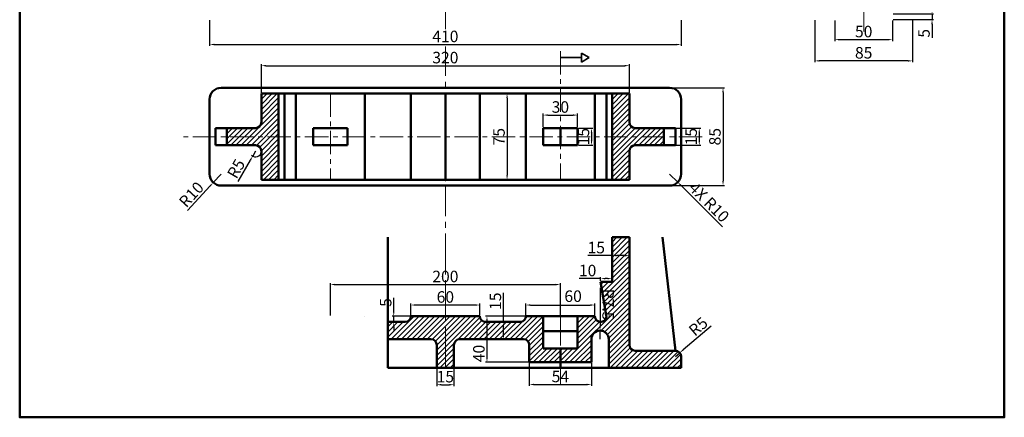
# Model space of a CAD drawing. Units: millimetres. Extents: x -150 to 761, y -175 to 827.
# Tile 1 of 2: x -95 to 761, y -175 to 171. Entities that reach past the tile are written whole.
import ezdxf

# ---------------------------------------------------------------- set-up
doc = ezdxf.new("R2010")
doc.units = ezdxf.units.MM
doc.header["$LTSCALE"] = 0.8
for name, pattern in [('CENTER', [50.8, 31.75, -6.35, 6.35, -6.35]), ('HIDDEN', [9.525, 6.35, -3.175]), ('PHANTOM', [63.5, 31.75, -6.35, 6.35, -6.35, 6.35, -6.35])]:
    doc.linetypes.add(name, pattern=pattern)
for name, color, linetype, lineweight in [('M-CNTR', 1, 'CENTER', 18), ('M-DIMS', 2, 'Continuous', 25), ('M-HATC', 8, 'Continuous', 18), ('M-HIDN', 4, 'HIDDEN', 25), ('M-OUTL', 7, 'Continuous', 50), ('M-SECT', 6, 'PHANTOM', 35), ('M-TTLB', 7, 'Continuous', 50)]:
    doc.layers.add(name, color=color, linetype=linetype, lineweight=lineweight)
doc.styles.get("Standard").update_dxf_attribs({"font": 'arial.ttf'})
doc.dimstyles.new('ISO-25', dxfattribs={"dimtxt": 10, "dimasz": 4, "dimexe": 1.25, "dimexo": 0.625, "dimtad": 1, "dimtxsty": 'Standard', "dimcen": 2.5, "dimadec": 0, "dimazin": 0, "dimtfac": 1, "dimtmove": 0, "dimatfit": 3, "dimfxl": 1, "dimarcsym": 0})

# ---------------------------------------------------------------- blocks, each defined once
blk = doc.blocks.new('*U1')
at = {"layer": 'M-CNTR', "color": 0, "transparency": 16777216}
blk.add_line((0, -217.92), (0, 196), dxfattribs=at)
blk = doc.blocks.new('*D9')
at = {"layer": 'Defpoints', "color": 0, "transparency": 16777216}
for p in [(663.68, 175.67), (663.68, 170.67), (698.09, 170.67)]:
    blk.add_point(p, dxfattribs=at)
at = {"layer": 'M-DIMS', "color": 0, "lineweight": -2, "transparency": 16777216}
for p, q in [((698.09, 179.67), (698.09, 183.67)), ((664.3, 175.67), (699.34, 175.67)), ((698.09, 175.67), (698.09, 170.67)), ((664.3, 170.67), (699.34, 170.67)), ((698.09, 166.67), (698.09, 154.79))]:
    blk.add_line(p, q, dxfattribs=at)
at = {"layer": 'M-DIMS', "color": 0, "transparency": 16777216}
for points in [[(697.42, 179.67), (698.75, 179.67), (698.09, 175.67)], [(697.42, 166.67), (698.75, 166.67), (698.09, 170.67)]]:
    blk.add_solid(points, dxfattribs=at)
at = {"layer": 'M-DIMS', "color": 0, "transparency": 16777216, "insert": (692.38, 158.73), "char_height": 10, "attachment_point": 5, "rotation": 90}
blk.add_mtext('5', dxfattribs=at)
blk = doc.blocks.new('*D10')
at = {"layer": 'Defpoints', "color": 0, "transparency": 16777216}
for p in [(613.68, 170.49), (663.68, 170.49), (663.68, 153.25)]:
    blk.add_point(p, dxfattribs=at)
at = {"layer": 'M-DIMS', "color": 0, "lineweight": -2, "transparency": 16777216}
for p, q in [((613.68, 169.87), (613.68, 152)), ((663.68, 169.87), (663.68, 152)), ((617.68, 153.25), (659.68, 153.25))]:
    blk.add_line(p, q, dxfattribs=at)
at = {"layer": 'M-DIMS', "color": 0, "transparency": 16777216}
for points in [[(617.68, 153.91), (617.68, 152.58), (613.68, 153.25)], [(659.68, 153.91), (659.68, 152.58), (663.68, 153.25)]]:
    blk.add_solid(points, dxfattribs=at)
at = {"layer": 'M-DIMS', "color": 0, "transparency": 16777216, "insert": (638.68, 158.98), "char_height": 10, "attachment_point": 5}
blk.add_mtext('50', dxfattribs=at)
blk = doc.blocks.new('*D11')
at = {"layer": 'Defpoints', "color": 0, "transparency": 16777216}
for p in [(596.18, 170.67), (681.18, 170.67), (596.18, 134.79)]:
    blk.add_point(p, dxfattribs=at)
at = {"layer": 'M-DIMS', "color": 0, "lineweight": -2, "transparency": 16777216}
for p, q in [((596.18, 170.04), (596.18, 133.54)), ((681.18, 170.04), (681.18, 133.54)), ((677.18, 134.79), (600.18, 134.79))]:
    blk.add_line(p, q, dxfattribs=at)
at = {"layer": 'M-DIMS', "color": 0, "transparency": 16777216}
for points in [[(600.18, 135.45), (600.18, 134.12), (596.18, 134.79)], [(677.18, 135.45), (677.18, 134.12), (681.18, 134.79)]]:
    blk.add_solid(points, dxfattribs=at)
at = {"layer": 'M-DIMS', "color": 0, "transparency": 16777216, "insert": (638.68, 140.52), "char_height": 10, "attachment_point": 5}
blk.add_mtext('85', dxfattribs=at)
blk = doc.blocks.new('*D19')
at = {"layer": 'Defpoints', "color": 0, "ltscale": 0.8, "transparency": 16777216}
for p in [(69.95, 170.67), (479.95, 170.67), (479.95, 149.01)]:
    blk.add_point(p, dxfattribs=at)
at = {"layer": 'M-DIMS', "color": 0, "lineweight": -2, "ltscale": 0.8, "transparency": 16777216}
for p, q in [((69.95, 170.04), (69.95, 147.76)), ((479.95, 170.04), (479.95, 147.76)), ((73.95, 149.01), (475.95, 149.01))]:
    blk.add_line(p, q, dxfattribs=at)
at = {"layer": 'M-DIMS', "color": 0, "ltscale": 0.8, "transparency": 16777216}
for points in [[(73.95, 149.68), (73.95, 148.35), (69.95, 149.01)], [(475.95, 149.68), (475.95, 148.35), (479.95, 149.01)]]:
    blk.add_solid(points, dxfattribs=at)
at = {"layer": 'M-DIMS', "color": 0, "ltscale": 0.8, "transparency": 16777216, "insert": (274.95, 154.74), "char_height": 10, "attachment_point": 5}
blk.add_mtext('410', dxfattribs=at)
blk = doc.blocks.new('*D28')
at = {"layer": 'Defpoints', "color": 0, "ltscale": 0.8, "transparency": 16777216}
for p in [(434.95, 130.61), (114.95, 106.4), (434.95, 106.4)]:
    blk.add_point(p, dxfattribs=at)
at = {"layer": 'M-DIMS', "color": 0, "lineweight": -2, "ltscale": 0.8, "transparency": 16777216}
for p, q in [((114.95, 107.03), (114.95, 131.86)), ((118.95, 130.61), (430.95, 130.61)), ((434.95, 107.03), (434.95, 131.86))]:
    blk.add_line(p, q, dxfattribs=at)
at = {"layer": 'M-DIMS', "color": 0, "ltscale": 0.8, "transparency": 16777216}
for points in [[(118.95, 131.28), (118.95, 129.95), (114.95, 130.61)], [(430.95, 131.28), (430.95, 129.95), (434.95, 130.61)]]:
    blk.add_solid(points, dxfattribs=at)
at = {"layer": 'M-DIMS', "color": 0, "ltscale": 0.8, "transparency": 16777216, "insert": (274.95, 136.35), "char_height": 10, "attachment_point": 5}
blk.add_mtext('320', dxfattribs=at)
blk = doc.blocks.new('*D29')
at = {"layer": 'Defpoints', "color": 0, "ltscale": 0.8, "transparency": 16777216}
for p in [(389.95, 87.67), (359.95, 76.4), (389.95, 76.4)]:
    blk.add_point(p, dxfattribs=at)
at = {"layer": 'M-DIMS', "color": 0, "lineweight": -2, "ltscale": 0.8, "transparency": 16777216}
for p, q in [((359.95, 77.03), (359.95, 88.92)), ((363.95, 87.67), (385.95, 87.67)), ((389.95, 77.03), (389.95, 88.92))]:
    blk.add_line(p, q, dxfattribs=at)
at = {"layer": 'M-DIMS', "color": 0, "ltscale": 0.8, "transparency": 16777216}
for points in [[(363.95, 88.34), (363.95, 87), (359.95, 87.67)], [(385.95, 88.34), (385.95, 87), (389.95, 87.67)]]:
    blk.add_solid(points, dxfattribs=at)
at = {"layer": 'M-DIMS', "color": 0, "ltscale": 0.8, "transparency": 16777216, "insert": (374.95, 93.4), "char_height": 10, "attachment_point": 5}
blk.add_mtext('30', dxfattribs=at)
blk = doc.blocks.new('*D30')
at = {"layer": 'Defpoints', "color": 0, "ltscale": 0.8, "transparency": 16777216}
for p in [(389.95, 76.4), (389.95, 61.4), (402.03, 61.4)]:
    blk.add_point(p, dxfattribs=at)
at = {"layer": 'M-DIMS', "color": 0, "lineweight": -2, "ltscale": 0.8, "transparency": 16777216}
for p, q in [((390.58, 76.4), (403.28, 76.4)), ((402.03, 72.4), (402.03, 65.4)), ((390.58, 61.4), (403.28, 61.4))]:
    blk.add_line(p, q, dxfattribs=at)
at = {"layer": 'M-DIMS', "color": 0, "ltscale": 0.8, "transparency": 16777216}
for points in [[(401.37, 72.4), (402.7, 72.4), (402.03, 76.4)], [(401.37, 65.4), (402.7, 65.4), (402.03, 61.4)]]:
    blk.add_solid(points, dxfattribs=at)
at = {"layer": 'M-DIMS', "color": 0, "ltscale": 0.8, "transparency": 16777216, "insert": (396.3, 68.9), "char_height": 10, "attachment_point": 5, "rotation": 90}
blk.add_mtext('15', dxfattribs=at)
blk = doc.blocks.new('*D31')
at = {"layer": 'Defpoints', "color": 0, "ltscale": 0.8, "transparency": 16777216}
for p in [(335.71, 106.4), (328.6, 31.4), (335.71, 31.4)]:
    blk.add_point(p, dxfattribs=at)
at = {"layer": 'M-DIMS', "color": 0, "lineweight": -2, "ltscale": 0.8, "transparency": 16777216}
for p, q in [((335.08, 106.4), (327.35, 106.4)), ((328.6, 102.4), (328.6, 35.4)), ((335.08, 31.4), (327.35, 31.4))]:
    blk.add_line(p, q, dxfattribs=at)
at = {"layer": 'M-DIMS', "color": 0, "ltscale": 0.8, "transparency": 16777216}
for points in [[(327.94, 102.4), (329.27, 102.4), (328.6, 106.4)], [(327.94, 35.4), (329.27, 35.4), (328.6, 31.4)]]:
    blk.add_solid(points, dxfattribs=at)
at = {"layer": 'M-DIMS', "color": 0, "ltscale": 0.8, "transparency": 16777216, "insert": (322.89, 68.9), "char_height": 10, "attachment_point": 5, "rotation": 90}
blk.add_mtext('75', dxfattribs=at)
blk = doc.blocks.new('*D32')
at = {"layer": 'Defpoints', "color": 0, "ltscale": 0.8, "transparency": 16777216}
for p in [(107.45, 52.07), (109.95, 56.4)]:
    blk.add_point(p, dxfattribs=at)
at = {"layer": 'M-DIMS', "color": 0, "lineweight": -2, "ltscale": 0.8, "transparency": 16777216}
for p, q in [((109.95, 56.4), (107.45, 52.07)), ((94.73, 30.03), (105.45, 48.61))]:
    blk.add_line(p, q, dxfattribs=at)
blk.add_arc((109.95, 56.4), 5, 225.67606, 352.83803, dxfattribs=at)
at = {"layer": 'M-DIMS', "color": 0, "ltscale": 0.8, "transparency": 16777216}
blk.add_solid([(104.87, 48.94), (106.03, 48.27), (107.45, 52.07)], dxfattribs=at)
at = {"layer": 'M-DIMS', "color": 0, "ltscale": 0.8, "transparency": 16777216, "insert": (94.14, 40.44), "char_height": 10, "attachment_point": 5, "rotation": 60}
blk.add_mtext('R5', dxfattribs=at)
blk = doc.blocks.new('*D33')
at = {"layer": 'Defpoints', "color": 0, "ltscale": 0.8, "transparency": 16777216}
for p in [(79.95, 36.4), (73.18, 29.04)]:
    blk.add_point(p, dxfattribs=at)
at = {"layer": 'M-DIMS', "color": 0, "lineweight": -2, "ltscale": 0.8, "transparency": 16777216}
for p, q in [((79.95, 36.4), (73.18, 29.04)), ((50.78, 4.66), (70.48, 26.09))]:
    blk.add_line(p, q, dxfattribs=at)
at = {"layer": 'M-DIMS', "color": 0, "ltscale": 0.8, "transparency": 16777216}
blk.add_solid([(69.99, 26.54), (70.97, 25.64), (73.18, 29.04)], dxfattribs=at)
at = {"layer": 'M-DIMS', "color": 0, "ltscale": 0.8, "transparency": 16777216, "insert": (55.05, 17.78), "char_height": 10, "attachment_point": 5, "rotation": 47.4138}
blk.add_mtext('R10', dxfattribs=at)
blk = doc.blocks.new('*D34')
at = {"layer": 'Defpoints', "color": 0, "ltscale": 0.8, "transparency": 16777216}
for p in [(457.45, 76.4), (457.45, 61.4), (495.7, 61.4)]:
    blk.add_point(p, dxfattribs=at)
at = {"layer": 'M-DIMS', "color": 0, "lineweight": -2, "ltscale": 0.8, "transparency": 16777216}
for p, q in [((458.08, 76.4), (496.95, 76.4)), ((495.7, 72.4), (495.7, 65.4)), ((458.08, 61.4), (496.95, 61.4))]:
    blk.add_line(p, q, dxfattribs=at)
at = {"layer": 'M-DIMS', "color": 0, "ltscale": 0.8, "transparency": 16777216}
for points in [[(495.03, 72.4), (496.37, 72.4), (495.7, 76.4)], [(495.03, 65.4), (496.37, 65.4), (495.7, 61.4)]]:
    blk.add_solid(points, dxfattribs=at)
at = {"layer": 'M-DIMS', "color": 0, "ltscale": 0.8, "transparency": 16777216, "insert": (489.97, 68.9), "char_height": 10, "attachment_point": 5, "rotation": 90}
blk.add_mtext('15', dxfattribs=at)
blk = doc.blocks.new('*D35')
at = {"layer": 'Defpoints', "color": 0, "ltscale": 0.8, "transparency": 16777216}
for p in [(454.34, 111.4), (454.34, 26.4), (516.37, 26.4)]:
    blk.add_point(p, dxfattribs=at)
at = {"layer": 'M-DIMS', "color": 0, "lineweight": -2, "ltscale": 0.8, "transparency": 16777216}
for p, q in [((454.96, 111.4), (517.62, 111.4)), ((516.37, 107.4), (516.37, 30.4)), ((454.96, 26.4), (517.62, 26.4))]:
    blk.add_line(p, q, dxfattribs=at)
at = {"layer": 'M-DIMS', "color": 0, "ltscale": 0.8, "transparency": 16777216}
for points in [[(515.7, 107.4), (517.03, 107.4), (516.37, 111.4)], [(515.7, 30.4), (517.03, 30.4), (516.37, 26.4)]]:
    blk.add_solid(points, dxfattribs=at)
at = {"layer": 'M-DIMS', "color": 0, "ltscale": 0.8, "transparency": 16777216, "insert": (510.64, 68.9), "char_height": 10, "attachment_point": 5, "rotation": 90}
blk.add_mtext('85', dxfattribs=at)
blk = doc.blocks.new('*D36')
at = {"layer": 'Defpoints', "color": 0, "ltscale": 0.8, "transparency": 16777216}
for p in [(404.95, -77.41), (344.95, -87.12), (404.95, -87.12)]:
    blk.add_point(p, dxfattribs=at)
at = {"layer": 'M-DIMS', "color": 0, "lineweight": -2, "ltscale": 0.8, "transparency": 16777216}
for p, q in [((344.95, -86.5), (344.95, -76.16)), ((404.95, -86.5), (404.95, -76.16)), ((348.95, -77.41), (400.95, -77.41))]:
    blk.add_line(p, q, dxfattribs=at)
at = {"layer": 'M-DIMS', "color": 0, "ltscale": 0.8, "transparency": 16777216}
for points in [[(348.95, -76.74), (348.95, -78.08), (344.95, -77.41)], [(400.95, -76.74), (400.95, -78.08), (404.95, -77.41)]]:
    blk.add_solid(points, dxfattribs=at)
at = {"layer": 'M-DIMS', "color": 0, "ltscale": 0.8, "transparency": 16777216, "insert": (386.01, -71.03), "char_height": 10, "attachment_point": 5}
blk.add_mtext('60', dxfattribs=at)
blk = doc.blocks.new('*D37')
at = {"layer": 'Defpoints', "color": 0, "ltscale": 0.8, "transparency": 16777216}
for p in [(244.95, -77.41), (244.95, -87.12), (304.95, -87.12)]:
    blk.add_point(p, dxfattribs=at)
at = {"layer": 'M-DIMS', "color": 0, "lineweight": -2, "ltscale": 0.8, "transparency": 16777216}
for p, q in [((244.95, -86.5), (244.95, -76.16)), ((304.95, -86.5), (304.95, -76.16)), ((300.95, -77.41), (248.95, -77.41))]:
    blk.add_line(p, q, dxfattribs=at)
at = {"layer": 'M-DIMS', "color": 0, "ltscale": 0.8, "transparency": 16777216}
for points in [[(248.95, -76.74), (248.95, -78.08), (244.95, -77.41)], [(300.95, -76.74), (300.95, -78.08), (304.95, -77.41)]]:
    blk.add_solid(points, dxfattribs=at)
at = {"layer": 'M-DIMS', "color": 0, "ltscale": 0.8, "transparency": 16777216, "insert": (274.95, -71.68), "char_height": 10, "attachment_point": 5}
blk.add_mtext('60', dxfattribs=at)
blk = doc.blocks.new('*D38')
at = {"layer": 'Defpoints', "color": 0, "ltscale": 0.8, "transparency": 16777216}
for p in [(230.05, -87.12), (232.45, -92.12), (252.9, -87.12)]:
    blk.add_point(p, dxfattribs=at)
at = {"layer": 'M-DIMS', "color": 0, "lineweight": -2, "ltscale": 0.8, "transparency": 16777216}
for p, q in [((230.05, -83.12), (230.05, -71.24)), ((252.27, -87.12), (228.8, -87.12)), ((231.83, -92.12), (228.8, -92.12)), ((230.05, -92.12), (230.05, -87.12)), ((230.05, -96.12), (230.05, -100.12))]:
    blk.add_line(p, q, dxfattribs=at)
at = {"layer": 'M-DIMS', "color": 0, "ltscale": 0.8, "transparency": 16777216}
for points in [[(229.39, -83.12), (230.72, -83.12), (230.05, -87.12)], [(229.39, -96.12), (230.72, -96.12), (230.05, -92.12)]]:
    blk.add_solid(points, dxfattribs=at)
at = {"layer": 'M-DIMS', "color": 0, "ltscale": 0.8, "transparency": 16777216, "insert": (224.34, -75.18), "char_height": 10, "attachment_point": 5, "rotation": 90}
blk.add_mtext('5', dxfattribs=at)
blk = doc.blocks.new('*D39')
at = {"layer": 'Defpoints', "color": 0, "ltscale": 0.8, "transparency": 16777216}
for p in [(374.95, -59.63), (174.95, -87.12), (374.95, -87.12)]:
    blk.add_point(p, dxfattribs=at)
at = {"layer": 'M-DIMS', "color": 0, "lineweight": -2, "ltscale": 0.8, "transparency": 16777216}
for p, q in [((174.95, -86.5), (174.95, -58.38)), ((178.95, -59.63), (370.95, -59.63)), ((374.95, -86.5), (374.95, -58.38))]:
    blk.add_line(p, q, dxfattribs=at)
at = {"layer": 'M-DIMS', "color": 0, "ltscale": 0.8, "transparency": 16777216}
for points in [[(178.95, -58.96), (178.95, -60.29), (174.95, -59.63)], [(370.95, -58.96), (370.95, -60.29), (374.95, -59.63)]]:
    blk.add_solid(points, dxfattribs=at)
at = {"layer": 'M-DIMS', "color": 0, "ltscale": 0.8, "transparency": 16777216, "insert": (274.95, -53.9), "char_height": 10, "attachment_point": 5}
blk.add_mtext('200', dxfattribs=at)
blk = doc.blocks.new('*D40')
at = {"layer": 'Defpoints', "color": 0, "ltscale": 0.8, "transparency": 16777216}
for p in [(324.95, -92.12), (324.95, -107.12), (325.45, -107.12)]:
    blk.add_point(p, dxfattribs=at)
at = {"layer": 'M-DIMS', "color": 0, "lineweight": -2, "ltscale": 0.8, "transparency": 16777216}
for p, q in [((325.45, -92.12), (325.45, -66.72)), ((325.58, -92.12), (326.7, -92.12)), ((325.45, -103.12), (325.45, -96.12)), ((325.58, -107.12), (326.7, -107.12))]:
    blk.add_line(p, q, dxfattribs=at)
at = {"layer": 'M-DIMS', "color": 0, "ltscale": 0.8, "transparency": 16777216}
for points in [[(324.79, -96.12), (326.12, -96.12), (325.45, -92.12)], [(324.79, -103.12), (326.12, -103.12), (325.45, -107.12)]]:
    blk.add_solid(points, dxfattribs=at)
at = {"layer": 'M-DIMS', "color": 0, "ltscale": 0.8, "transparency": 16777216, "insert": (319.72, -74.08), "char_height": 10, "attachment_point": 5, "rotation": 90}
blk.add_mtext('15', dxfattribs=at)
blk = doc.blocks.new('*D41')
at = {"layer": 'Defpoints', "color": 0, "ltscale": 0.8, "transparency": 16777216}
for p in [(349.36, -87.12), (311.12, -127.12), (353.08, -127.12)]:
    blk.add_point(p, dxfattribs=at)
at = {"layer": 'M-DIMS', "color": 0, "lineweight": -2, "ltscale": 0.8, "transparency": 16777216}
for p, q in [((348.74, -87.12), (309.87, -87.12)), ((311.12, -91.12), (311.12, -123.12)), ((352.45, -127.12), (309.87, -127.12))]:
    blk.add_line(p, q, dxfattribs=at)
at = {"layer": 'M-DIMS', "color": 0, "ltscale": 0.8, "transparency": 16777216}
for points in [[(310.45, -91.12), (311.79, -91.12), (311.12, -87.12)], [(310.45, -123.12), (311.79, -123.12), (311.12, -127.12)]]:
    blk.add_solid(points, dxfattribs=at)
at = {"layer": 'M-DIMS', "color": 0, "ltscale": 0.8, "transparency": 16777216, "insert": (305.39, -119.55), "char_height": 10, "attachment_point": 5, "rotation": 90}
blk.add_mtext('40', dxfattribs=at)
blk = doc.blocks.new('*D42')
at = {"layer": 'Defpoints', "color": 0, "ltscale": 0.8, "transparency": 16777216}
for p in [(347.95, -127.12), (401.95, -127.12), (401.95, -146.51)]:
    blk.add_point(p, dxfattribs=at)
at = {"layer": 'M-DIMS', "color": 0, "lineweight": -2, "ltscale": 0.8, "transparency": 16777216}
for p, q in [((347.95, -127.75), (347.95, -147.76)), ((401.95, -127.75), (401.95, -147.76)), ((351.95, -146.51), (397.95, -146.51))]:
    blk.add_line(p, q, dxfattribs=at)
at = {"layer": 'M-DIMS', "color": 0, "ltscale": 0.8, "transparency": 16777216}
for points in [[(351.95, -145.84), (351.95, -147.18), (347.95, -146.51)], [(397.95, -145.84), (397.95, -147.18), (401.95, -146.51)]]:
    blk.add_solid(points, dxfattribs=at)
at = {"layer": 'M-DIMS', "color": 0, "ltscale": 0.8, "transparency": 16777216, "insert": (374.95, -140.8), "char_height": 10, "attachment_point": 5}
blk.add_mtext('54', dxfattribs=at)
blk = doc.blocks.new('*D43')
at = {"layer": 'Defpoints', "color": 0, "ltscale": 0.8, "transparency": 16777216}
for p in [(409.95, -57.12), (419.95, -54.45), (419.95, -57.12)]:
    blk.add_point(p, dxfattribs=at)
at = {"layer": 'M-DIMS', "color": 0, "lineweight": -2, "ltscale": 0.8, "transparency": 16777216}
for p, q in [((409.95, -54.45), (391.35, -54.45)), ((409.95, -56.5), (409.95, -53.2)), ((415.95, -54.45), (413.95, -54.45)), ((419.95, -56.5), (419.95, -53.2))]:
    blk.add_line(p, q, dxfattribs=at)
at = {"layer": 'M-DIMS', "color": 0, "ltscale": 0.8, "transparency": 16777216}
for points in [[(413.95, -53.79), (413.95, -55.12), (409.95, -54.45)], [(415.95, -53.79), (415.95, -55.12), (419.95, -54.45)]]:
    blk.add_solid(points, dxfattribs=at)
at = {"layer": 'M-DIMS', "color": 0, "ltscale": 0.8, "transparency": 16777216, "insert": (398.65, -48.72), "char_height": 10, "attachment_point": 5}
blk.add_mtext('10', dxfattribs=at)
blk = doc.blocks.new('*D44')
at = {"layer": 'Defpoints', "color": 0, "ltscale": 0.8, "transparency": 16777216}
for p in [(419.95, -37.81), (434.95, -34.5), (434.95, -37.81)]:
    blk.add_point(p, dxfattribs=at)
at = {"layer": 'M-DIMS', "color": 0, "lineweight": -2, "ltscale": 0.8, "transparency": 16777216}
for p, q in [((419.95, -37.19), (419.95, -33.25)), ((434.95, -37.19), (434.95, -33.25)), ((419.95, -34.5), (398.8, -34.5)), ((430.95, -34.5), (423.95, -34.5))]:
    blk.add_line(p, q, dxfattribs=at)
at = {"layer": 'M-DIMS', "color": 0, "ltscale": 0.8, "transparency": 16777216}
for points in [[(423.95, -33.83), (423.95, -35.17), (419.95, -34.5)], [(430.95, -33.83), (430.95, -35.17), (434.95, -34.5)]]:
    blk.add_solid(points, dxfattribs=at)
at = {"layer": 'M-DIMS', "color": 0, "ltscale": 0.8, "transparency": 16777216, "insert": (406.15, -28.77), "char_height": 10, "attachment_point": 5}
blk.add_mtext('15', dxfattribs=at)
blk = doc.blocks.new('*D45')
at = {"layer": 'Defpoints', "color": 0, "ltscale": 0.8, "transparency": 16777216}
for p in [(478.76, -118.89), (474.95, -122.12)]:
    blk.add_point(p, dxfattribs=at)
at = {"layer": 'M-DIMS', "color": 0, "lineweight": -2, "ltscale": 0.8, "transparency": 16777216}
for p, q in [((506.01, -95.77), (481.81, -116.3)), ((474.95, -122.12), (478.76, -118.89))]:
    blk.add_line(p, q, dxfattribs=at)
at = {"layer": 'M-DIMS', "color": 0, "ltscale": 0.8, "transparency": 16777216}
blk.add_solid([(481.38, -115.79), (482.24, -116.81), (478.76, -118.89)], dxfattribs=at)
at = {"layer": 'M-DIMS', "color": 0, "ltscale": 0.8, "transparency": 16777216, "insert": (495.66, -97.06), "char_height": 10, "attachment_point": 5, "rotation": 40.31036}
blk.add_mtext('R5', dxfattribs=at)
blk = doc.blocks.new('*D46')
at = {"layer": 'Defpoints', "color": 0, "ltscale": 0.8, "transparency": 16777216}
for p in [(267.45, -132.12), (282.45, -132.12), (282.45, -146.7)]:
    blk.add_point(p, dxfattribs=at)
at = {"layer": 'M-DIMS', "color": 0, "lineweight": -2, "ltscale": 0.8, "transparency": 16777216}
for p, q in [((267.45, -132.75), (267.45, -147.95)), ((282.45, -132.75), (282.45, -147.95)), ((271.45, -146.7), (278.45, -146.7))]:
    blk.add_line(p, q, dxfattribs=at)
at = {"layer": 'M-DIMS', "color": 0, "ltscale": 0.8, "transparency": 16777216}
for points in [[(271.45, -146.03), (271.45, -147.37), (267.45, -146.7)], [(278.45, -146.03), (278.45, -147.37), (282.45, -146.7)]]:
    blk.add_solid(points, dxfattribs=at)
at = {"layer": 'M-DIMS', "color": 0, "ltscale": 0.8, "transparency": 16777216, "insert": (274.95, -140.97), "char_height": 10, "attachment_point": 5}
blk.add_mtext('15', dxfattribs=at)
blk = doc.blocks.new('*D54')
at = {"layer": 'Defpoints', "color": 0, "ltscale": 0.8, "transparency": 16777216}
for p in [(469.95, 36.4), (477.02, 29.33)]:
    blk.add_point(p, dxfattribs=at)
at = {"layer": 'M-DIMS', "color": 0, "lineweight": -2, "ltscale": 0.8, "transparency": 16777216}
for p, q in [((469.95, 36.4), (477.02, 29.33)), ((515.91, -9.56), (479.85, 26.5))]:
    blk.add_line(p, q, dxfattribs=at)
at = {"layer": 'M-DIMS', "color": 0, "ltscale": 0.8, "transparency": 16777216}
blk.add_solid([(480.32, 26.97), (479.38, 26.03), (477.02, 29.33)], dxfattribs=at)
at = {"layer": 'M-DIMS', "color": 0, "ltscale": 0.8, "transparency": 16777216, "insert": (503.35, 11.11), "char_height": 10, "attachment_point": 5, "rotation": 314.99833}
blk.add_mtext('4X R10', dxfattribs=at)
blk = doc.blocks.new('*D55')
at = {"layer": 'Defpoints', "color": 0, "ltscale": 0.8, "transparency": 16777216}
for p in [(409.45, -99.62), (409.45, -107.12)]:
    blk.add_point(p, dxfattribs=at)
at = {"layer": 'M-DIMS', "color": 0, "lineweight": -2, "ltscale": 0.8, "transparency": 16777216}
for p, q in [((409.45, -62.52), (409.45, -95.62)), ((409.45, -107.12), (409.45, -99.62))]:
    blk.add_line(p, q, dxfattribs=at)
at = {"layer": 'M-DIMS', "color": 0, "ltscale": 0.8, "transparency": 16777216}
blk.add_solid([(410.12, -95.62), (408.78, -95.62), (409.45, -99.62)], dxfattribs=at)
at = {"layer": 'M-DIMS', "color": 0, "ltscale": 0.8, "transparency": 16777216, "insert": (415.16, -77.07), "char_height": 10, "attachment_point": 5, "rotation": 270.00235}
blk.add_mtext('R7.5', dxfattribs=at)

msp = doc.modelspace()

# ---------------------------------------------------------------- hatches: boundary and pattern name
at = {"layer": 'M-HATC', "ltscale": 0.8}
h = msp.add_hatch(dxfattribs=at)
h.set_pattern_fill('ANSI31', color=256)
h.paths.add_polyline_path([(129.95, 106.4), (114.95, 106.4), (114.95, 81.4, -0.4142136), (109.95, 76.4), (84.95, 76.4), (84.95, 68.9), (129.95, 68.9)])
h.paths.add_polyline_path([(129.95, 68.9), (84.95, 68.9), (84.95, 61.4), (109.95, 61.4, -0.4142136), (114.95, 56.4), (114.95, 31.4), (129.95, 31.4)])
h.paths.add_polyline_path([(434.95, 81.4), (434.95, 106.4), (419.95, 106.4), (419.95, 68.9), (464.95, 68.9), (464.95, 76.4), (439.95, 76.4, -0.4142136)])
h.paths.add_polyline_path([(439.95, 61.4), (464.95, 61.4), (464.95, 68.9), (419.95, 68.9), (419.95, 31.4), (434.95, 31.4), (434.95, 56.4, -0.4142136)])
h = msp.add_hatch(dxfattribs=at)
h.set_pattern_fill('ANSI31', color=256)
h.set_pattern_definition([(45, (-1269.3077, -162.8122), (-2.245064, 2.245064), [])])
h.paths.add_polyline_path([(359.95, -87.121), (344.95, -87.121, -0.4142136), (339.95, -92.121), (309.95, -92.121, -0.4142136), (304.95, -87.121), (274.95, -87.121), (274.95, -132.121), (282.45, -132.121), (282.45, -112.121, -0.4142136), (287.45, -107.121), (342.95, -107.121, -0.4142136), (347.95, -112.121), (347.95, -127.121), (374.95, -127.121), (374.95, -115.121), (359.95, -115.121)])
h.paths.add_polyline_path([(274.95, -87.121), (244.95, -87.121, -0.4142136), (239.95, -92.121), (224.95, -92.121), (224.95, -107.121), (262.45, -107.121, -0.4142136), (267.45, -112.121), (267.45, -132.121), (274.95, -132.121)])
h.paths.add_polyline_path([(401.95, -107.121, -1), (416.95, -107.121), (416.95, -132.121), (479.95, -132.121), (479.95, -122.121, 0.4142136), (474.95, -117.121), (439.95, -117.121, -0.4142136), (434.95, -112.121), (434.95, -18.503), (419.95, -18.503), (419.95, -57.121), (409.95, -57.121), (414.88, -86.288, -1.0874353), (404.95, -87.121), (389.95, -87.121), (389.95, -115.121), (374.95, -115.121), (374.95, -127.121), (401.95, -127.121)])

# ---------------------------------------------------------------- linework, layer by layer
at = {"layer": 'M-CNTR'}
for p, q in [((274.95, -122.062), (274.95, 589.539)), ((274.95, -132.121), (274.95, -18.503)), ((204.95, -87.121), (204.95, -87.121)), ((344.95, -87.121), (344.95, -87.121)), ((374.95, -87.121), (374.95, -146.16))]:
    msp.add_line(p, q, dxfattribs=at)
at = {"layer": 'M-CNTR', "ltscale": 0.8}
for p, q in [((374.95, 143.262), (374.95, 31.4)), ((174.95, 106.4), (174.95, 31.4)), ((498.33, 68.9), (45.612, 68.9))]:
    msp.add_line(p, q, dxfattribs=at)
at = {"layer": 'M-HIDN', "ltscale": 0.8}
msp.add_line((389.95, -87.121), (359.95, -87.121), dxfattribs=at)
at = {"layer": 'M-OUTL', "ltscale": 0.8}
for p, q in [((114.95, 106.4), (114.95, 81.4)), ((129.95, 106.4), (129.95, 31.4)), ((134.95, 106.4), (134.95, 31.4)), ((144.95, 106.4), (144.95, 31.4)), ((204.95, 106.4), (204.95, 31.4)), ((244.95, 106.4), (244.95, 31.4)), ((274.95, 106.4), (274.95, 31.4)), ((304.95, 106.4), (304.95, 31.4)), ((344.95, 106.4), (344.95, 31.4)), ((404.95, 106.4), (404.95, 31.4)), ((414.95, 106.4), (414.95, 31.4)), ((419.95, 106.4), (419.95, 31.4)), ((434.95, 106.4), (434.95, 81.4)), ((74.95, 76.4), (109.95, 76.4)), ((84.95, 76.4), (84.95, 61.4)), ((159.95, 61.4), (159.95, 76.4)), ((159.95, 76.4), (189.95, 76.4)), ((189.95, 76.4), (189.95, 61.4)), ((359.95, 76.4), (359.95, 61.4)), ((389.95, 76.4), (359.95, 76.4)), ((374.95, 76.4), (374.95, 61.4)), ((389.95, 61.4), (389.95, 76.4)), ((474.95, 76.4), (439.95, 76.4)), ((464.95, 76.4), (464.95, 61.4)), ((74.95, 61.4), (109.95, 61.4)), ((189.95, 61.4), (159.95, 61.4)), ((359.95, 61.4), (389.95, 61.4)), ((474.95, 61.4), (439.95, 61.4)), ((114.95, 56.4), (114.95, 31.4)), ((434.95, 56.4), (434.95, 31.4)), ((224.95, -18.503), (224.95, -132.121)), ((419.95, -18.503), (434.95, -18.503)), ((414.88, -86.288), (409.95, -57.121)), ((239.95, -92.121), (224.95, -92.121)), ((309.95, -92.121), (339.95, -92.121)), ((344.95, -87.121), (404.95, -87.121)), ((359.95, -87.121), (359.95, -115.121)), ((389.95, -115.121), (389.95, -87.121)), ((359.95, -100.121), (389.95, -100.121)), ((262.45, -107.121), (224.95, -107.121)), ((287.45, -107.121), (342.95, -107.121)), ((401.95, -107.121), (401.95, -127.121)), ((416.95, -107.121), (416.95, -132.121)), ((267.45, -132.121), (267.45, -112.121)), ((282.45, -132.121), (282.45, -112.121)), ((347.95, -112.121), (347.95, -127.121)), ((359.95, -115.121), (389.95, -115.121)), ((374.95, -115.121), (374.95, -132.121)), ((347.95, -127.121), (401.95, -127.121))]:
    msp.add_line(p, q, dxfattribs=at)
at = {"layer": 'M-OUTL'}
for p, q in [((419.95, -57.121), (419.95, -18.503)), ((434.95, -112.121), (434.95, -18.503)), ((463.731, -18.503), (474.95, -117.121)), ((409.95, -57.121), (419.95, -57.121)), ((244.95, -87.121), (304.95, -87.121)), ((244.95, -87.121), (244.95, -87.121)), ((304.95, -87.121), (304.95, -87.121)), ((474.95, -117.121), (439.95, -117.121)), ((479.95, -132.121), (479.95, -122.121)), ((224.95, -132.121), (479.95, -132.121))]:
    msp.add_line(p, q, dxfattribs=at)
msp.add_lwpolyline([(479.95, 101.4), (479.95, 36.4, -0.4142136), (469.95, 26.4), (79.95, 26.4, -0.4142136), (69.95, 36.4), (69.95, 101.4, -0.4142136), (79.95, 111.4), (469.95, 111.4, -0.4142136)], format="xyb", close=True, dxfattribs=at)
for points in [[(114.95, 106.4), (434.95, 106.4)], [(74.95, 61.4), (74.95, 76.4)], [(474.95, 61.4), (474.95, 76.4)], [(434.95, 31.4), (114.95, 31.4)]]:
    msp.add_lwpolyline(points, dxfattribs=at)
at = {"layer": 'M-OUTL', "ltscale": 0.8}
for centre, radius, start, end in [((109.95, 81.4), 5, 270, 0), ((439.95, 81.4), 5, 180, 270), ((109.95, 56.4), 5, 0, 90), ((439.95, 56.4), 5, 90, 180), ((309.95, -87.121), 5, 180, 270), ((339.95, -87.121), 5, 270, 0), ((409.95, -87.121), 5, 180, 9.594068), ((409.45, -107.121), 7.5, 0, 180), ((262.45, -112.121), 5, 0, 90), ((287.45, -112.121), 5, 90, 180), ((342.95, -112.121), 5, 0, 90), ((439.95, -112.121), 5, 180, 270)]:
    msp.add_arc(centre, radius, start, end, dxfattribs=at)
at = {"layer": 'M-OUTL'}
for centre, start, end in [((239.95, -87.121), 270, 0), ((474.95, -122.121), 0, 90)]:
    msp.add_arc(centre, 5, start, end, dxfattribs=at)
at = {"layer": 'M-SECT', "ltscale": 0.8}
for p, q in [((374.95, 137.663), (393.231, 137.663)), ((399.988, 137.663), (393.231, 141.564)), ((393.231, 133.761), (393.231, 141.564)), ((399.988, 137.663), (393.231, 133.761))]:
    msp.add_line(p, q, dxfattribs=at)
at = {"layer": 'M-TTLB', "ltscale": 0.8}
msp.add_lwpolyline([(-95.156, 653.208), (760.935, 653.208), (760.935, -175.003), (-95.156, -175.003)], close=True, dxfattribs=at)

# ---------------------------------------------------------------- block references
at = {"layer": 'M-CNTR'}
msp.add_blockref('*U1', (638.678, 378.17), dxfattribs=at)

# ---------------------------------------------------------------- dimensions: what is measured, and where the dimension line sits
at = {"layer": 'M-DIMS'}
dim = msp.add_linear_dim(base=(698.087, 170.67), p1=(663.678, 175.67), p2=(663.678, 170.67), angle=90, dimstyle='ISO-25', override={"dimclrd": 0, "dimclre": 0, "dimclrt": 0}, dxfattribs=at)
dim.commit()
dim.dimension.update_dxf_attribs({"geometry": '*D9', "text_midpoint": (692.377, 158.729)})
at = {"layer": 'M-DIMS', "ltscale": 0.8}
for base, p1, p2, picture, middle in [((479.95, 149.013), (69.95, 170.67), (479.95, 170.67), '*D19', (274.95, 154.744)), ((434.95, 130.612), (114.95, 106.4), (434.95, 106.4), '*D28', (274.95, 136.346)), ((389.95, 87.669), (359.95, 76.4), (389.95, 76.4), '*D29', (374.95, 93.403)), ((374.95, -59.626), (174.95, -87.121), (374.95, -87.121), '*D39', (274.95, -53.895)), ((401.95, -146.51), (347.95, -127.121), (401.95, -127.121), '*D42', (374.95, -140.8)), ((282.45, -146.7), (267.45, -132.121), (282.45, -132.121), '*D46', (274.95, -140.969))]:
    dim = msp.add_linear_dim(base=base, p1=p1, p2=p2, dimstyle='ISO-25', override={"dimclrd": 0, "dimclre": 0, "dimclrt": 0}, dxfattribs=at)
    dim.commit()
    dim.dimension.update_dxf_attribs({"geometry": picture, "text_midpoint": middle})
at = {"layer": 'M-DIMS'}
for base, p1, p2, picture, middle in [((596.178, 134.787), (681.178, 170.67), (596.178, 170.67), '*D11', (638.678, 140.518)), ((663.678, 153.248), (613.678, 170.493), (663.678, 170.493), '*D10', (638.678, 158.978))]:
    dim = msp.add_linear_dim(base=base, p1=p1, p2=p2, dimstyle='ISO-25', override={"dimclrd": 0, "dimclre": 0, "dimclrt": 0}, dxfattribs=at)
    dim.commit()
    dim.dimension.update_dxf_attribs({"geometry": picture, "text_midpoint": middle})
at = {"layer": 'M-DIMS', "ltscale": 0.8}
for base, p1, p2, picture, middle in [((516.367, 26.4), (454.339, 111.4), (454.339, 26.4), '*D35', (510.636, 68.9)), ((328.603, 31.4), (335.707, 106.4), (335.707, 31.4), '*D31', (322.893, 68.9)), ((402.032, 61.4), (389.95, 76.4), (389.95, 61.4), '*D30', (396.301, 68.9)), ((495.699, 61.4), (457.45, 76.4), (457.45, 61.4), '*D34', (489.969, 68.9)), ((230.052, -87.121), (232.45, -92.121), (252.9, -87.121), '*D38', (224.342, -75.181))]:
    dim = msp.add_linear_dim(base=base, p1=p1, p2=p2, angle=90, dimstyle='ISO-25', override={"dimclrd": 0, "dimclre": 0, "dimclrt": 0}, dxfattribs=at)
    dim.commit()
    dim.dimension.update_dxf_attribs({"geometry": picture, "text_midpoint": middle})
for center, mpoint, override, picture, middle in [((109.95, 56.4), (107.45, 52.07), {"dimclrd": 0, "dimclre": 0, "dimclrt": 0}, '*D32', (94.142, 40.441)), ((79.95, 36.4), (73.183, 29.038), {"dimclrd": 0, "dimclre": 0, "dimclrt": 0}, '*D33', (55.054, 17.781)), ((409.45, -107.121), (409.45, -99.621), {"dimdec": 1, "dimlfac": 1, "dimrnd": 0, "dimzin": 0, "dimdsep": 46, "dimlunit": 2}, '*D55', (415.159, -77.07))]:
    dim = msp.add_radius_dim(center=center, mpoint=mpoint, dimstyle='ISO-25', override=override, dxfattribs=at)
    dim.commit()
    dim.dimension.update_dxf_attribs({"geometry": picture, "text_midpoint": middle})
dim = msp.add_radius_dim(center=(469.95, 36.4), mpoint=(477.021, 29.329), text='4X <>', dimstyle='ISO-25', override={"dimdec": 0, "dimlfac": 1, "dimrnd": 0, "dimzin": 0, "dimdsep": 46, "dimlunit": 2}, dxfattribs=at)
dim.commit()
dim.dimension.update_dxf_attribs({"geometry": '*D54', "text_midpoint": (503.347, 11.106)})
for base, p1, p2, override, picture, middle in [((434.95, -34.5), (419.95, -37.812), (434.95, -37.812), {"dimclrd": 0, "dimclre": 0, "dimclrt": 0}, '*D44', (406.15, -34.5)), ((419.95, -54.453), (409.95, -57.121), (419.95, -57.121), {"dimclrd": 0, "dimclre": 0, "dimclrt": 0}, '*D43', (398.651, -54.453)), ((244.95, -77.409), (304.95, -87.121), (244.95, -87.121), {"dimclrd": 0, "dimclre": 0, "dimclrt": 0, "dimtmove": 0}, '*D37', (274.95, -77.409)), ((404.95, -77.409), (344.95, -87.121), (404.95, -87.121), {"dimclrd": 0, "dimclre": 0, "dimclrt": 0, "dimtmove": 2}, '*D36', (386.006, -71.026))]:
    dim = msp.add_linear_dim(base=base, p1=p1, p2=p2, dimstyle='ISO-25', override=override, dxfattribs=at)
    dim.commit()
    dim.dimension.update_dxf_attribs({"geometry": picture, "text_midpoint": middle, "dimtype": 160})
for base, p1, p2, picture, middle in [((325.454, -107.121), (324.95, -92.121), (324.95, -107.121), '*D40', (325.454, -74.079)), ((311.119, -127.121), (349.363, -87.121), (353.077, -127.121), '*D41', (311.119, -119.555))]:
    dim = msp.add_linear_dim(base=base, p1=p1, p2=p2, angle=90, dimstyle='ISO-25', override={"dimclrd": 0, "dimclre": 0, "dimclrt": 0}, dxfattribs=at)
    dim.commit()
    dim.dimension.update_dxf_attribs({"geometry": picture, "text_midpoint": middle, "dimtype": 160})
dim = msp.add_radius_dim(center=(474.95, -122.121), mpoint=(478.763, -118.887), dimstyle='ISO-25', override={"dimclrd": 0, "dimclre": 0, "dimclrt": 0}, dxfattribs=at)
dim.commit()
dim.dimension.update_dxf_attribs({"geometry": '*D45', "text_midpoint": (499.353, -101.419), "dimtype": 164})

doc.saveas('drawing.dxf')
